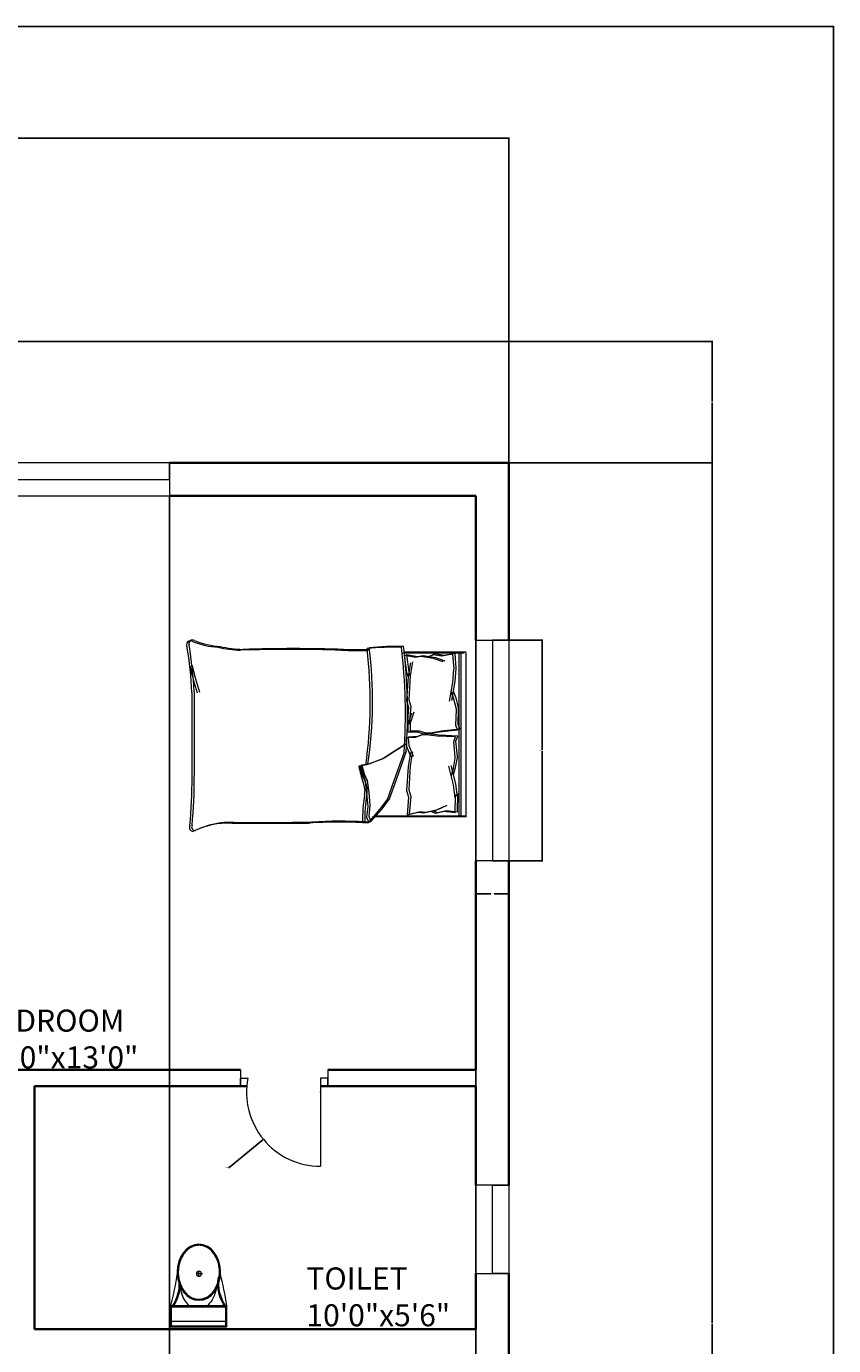
# Model space of a CAD drawing. Units: inches. Extents: x 1902 to 2626, y 1199 to 2408.
# Tile 9 of 9: x 2407 to 2626, y 2049 to 2408. Entities that reach past the tile are written whole.
import ezdxf

# ---------------------------------------------------------------- set-up
doc = ezdxf.new("R2010")
doc.units = ezdxf.units.IN
for name, color, linetype, lineweight in [('A-ANNO-DIMS', 2, 'Continuous', 18), ('A-ANNO-TTLB', 7, 'Continuous', 25), ('A-AREA-IDEN', 7, 'Continuous', 18), ('A-DOOR', 31, 'Continuous', 18), ('A-FLOR-FIXT', 9, 'Continuous', 18), ('A-FURN', 8, 'Continuous', 13), ('A-GLAZ', 181, 'Continuous', 18), ('A-WALL', 7, 'Continuous', 35)]:
    doc.layers.add(name, color=color, linetype=linetype, lineweight=lineweight)
doc.styles.get("Standard").update_dxf_attribs({"font": 'arial.ttf'})
doc.dimstyles.get("Standard").update_dxf_attribs({"dimtxt": 0.18, "dimasz": 0.18, "dimexe": 0.18, "dimexo": 0.0625, "dimgap": 0.09, "dimtad": 0, "dimtih": 1, "dimtoh": 1, "dimdec": 4, "dimzin": 0, "dimdsep": 46, "dimtxsty": 'Standard', "dimcen": 0.09, "dimadec": 0, "dimazin": 0, "dimtfac": 1, "dimtdec": 4, "dimtofl": 0, "dimtmove": 0, "dimatfit": 3, "dimfxl": 1, "dimtolj": 1, "dimtzin": 0, "dimarcsym": 0})

# ---------------------------------------------------------------- blocks, each defined once
blk = doc.blocks.new('A$C31115884')
for p, q in [((283, 498), (223, 498)), ((258, 466), (258, 523)), ((0, 200), (0, 0)), ((520, 200), (0, 200)), ((10, 190), (10, 10)), ((510, 190), (10, 190)), ((510, 10), (510, 190)), ((520, 0), (520, 200)), ((510, 54), (0, 54)), ((10, 10), (510, 10)), ((0, 0), (520, 0))]:
    blk.add_line(p, q)
blk.add_circle((256, 496), 23.6)
for centre, radius, start, end in [((2778, -205), 2807, 165.4549, 171.7133), ((3237, 905), 2807, 188.2867, 194.5451), ((-295, 403), 365, 324.2091, 9.3499), ((-295, 403), 375, 324.2091, 9.3499), ((139, 406), 293, 315.8436, 2.6563), ((806, 403), 375, 179.2036, 215.7909), ((806, 403), 365, 170.6501, 215.7909), ((384, 406), 293, 190.2774, 224.1564)]:
    blk.add_arc(centre, radius, start, end)
blk.add_ellipse((256, 510), major_axis=(0, -261), ratio=0.772727)
blk.add_open_spline([(256, 259), (263, 259), (270, 260), (288, 262), (299, 265), (320, 273), (330, 278), (350, 291), (360, 299), (378, 316), (386, 326), (402, 347), (409, 358), (421, 383), (427, 395), (436, 422), (440, 436), (445, 465), (447, 480), (448, 509), (448, 524), (445, 553), (443, 568), (436, 596), (432, 610), (422, 636), (416, 649), (402, 672), (395, 683), (379, 703), (370, 712), (351, 728), (341, 735), (321, 746), (310, 751), (289, 757), (278, 759), (256, 761), (245, 761), (223, 757), (212, 754), (191, 746), (181, 741), (161, 728), (151, 720), (133, 703), (125, 693), (110, 672), (103, 660), (90, 636), (85, 623), (76, 596), (72, 582), (67, 553), (66, 538), (64, 509), (65, 494), (68, 465), (70, 450), (77, 422), (81, 408), (91, 382), (97, 370), (111, 346), (118, 335), (135, 316), (144, 307), (162, 291), (172, 284), (193, 273), (203, 269), (225, 262), (236, 260), (250, 259), (253, 259), (256, 259)], degree=3, knots=[0, 0, 0, 0, 0.110105, 0.110105, 0.285049, 0.285049, 0.459994, 0.459994, 0.634938, 0.634938, 0.809882, 0.809882, 0.984827, 0.984827, 1.159771, 1.159771, 1.334715, 1.334715, 1.50966, 1.50966, 1.684604, 1.684604, 1.859549, 1.859549, 2.034493, 2.034493, 2.209437, 2.209437, 2.384382, 2.384382, 2.559326, 2.559326, 2.73427, 2.73427, 2.909215, 2.909215, 3.084159, 3.084159, 3.259103, 3.259103, 3.434048, 3.434048, 3.608992, 3.608992, 3.783936, 3.783936, 3.958881, 3.958881, 4.133825, 4.133825, 4.30877, 4.30877, 4.483714, 4.483714, 4.658658, 4.658658, 4.833603, 4.833603, 5.008547, 5.008547, 5.183491, 5.183491, 5.358436, 5.358436, 5.53338, 5.53338, 5.708324, 5.708324, 5.883269, 5.883269, 6.058213, 6.058213, 6.233158, 6.233158, 6.283185, 6.283185, 6.283185, 6.283185])
blk = doc.blocks.new('BED-DOUBLE')
for p, q in [((-0.01, 48.09), (0.59, 48.09)), ((-0.01, 48.09), (-0.01, 3.46)), ((-0.01, 47.87), (24.84, 47.87)), ((-0.01, 47.87), (24.84, 47.87)), ((0.59, 48.09), (25.44, 48.09)), ((0.59, 48.09), (25.44, 48.09)), ((1.43, 3.25), (1.43, 47.87)), ((1.43, 3.25), (1.43, 47.87)), ((2.02, 3.46), (2.02, 48.09)), ((2.02, 3.46), (2.02, 48.09)), ((2.38, 46.8), (2.29, 41.75)), ((2.38, 46.8), (2.29, 41.75)), ((2.38, 46.8), (5.38, 46.44)), ((2.38, 46.8), (5.38, 46.44)), ((2.98, 47.01), (2.89, 41.97)), ((2.98, 47.01), (2.89, 41.96)), ((2.98, 47.01), (5.98, 46.66)), ((2.98, 47.01), (5.98, 46.66)), ((5.38, 46.44), (7.78, 47)), ((5.38, 46.44), (7.78, 47)), ((5.98, 46.66), (8.38, 47.21)), ((5.98, 46.66), (8.38, 47.21)), ((11.04, 46.8), (7.7, 46.05)), ((11.04, 46.8), (7.7, 46.05)), ((7.78, 47), (8.76, 46.52)), ((7.78, 47), (8.76, 46.52)), ((11.64, 47.01), (8.3, 46.26)), ((11.64, 47.01), (8.3, 46.26)), ((8.38, 47.21), (9.35, 46.73)), ((8.38, 47.21), (9.35, 46.73)), ((12.54, 46.62), (11.04, 46.8)), ((12.54, 46.62), (11.04, 46.8)), ((13.14, 46.83), (11.64, 47.01)), ((13.14, 46.83), (11.64, 47.01)), ((15.47, 47.34), (12.54, 46.62)), ((15.47, 47.34), (12.54, 46.62)), ((16.07, 47.56), (13.14, 46.83)), ((16.07, 47.56), (13.14, 46.83)), ((15.09, 42.55), (15.47, 47.34)), ((15.09, 42.55), (15.47, 47.34)), ((15.69, 42.77), (16.07, 47.56)), ((15.69, 42.77), (16.07, 47.56)), ((25.9, 49.37), (22.87, 45.91)), ((25.9, 49.37), (22.87, 45.91)), ((26.5, 49.58), (23.46, 46.12)), ((26.5, 49.58), (23.46, 46.12)), ((27.53, 49.44), (25.9, 49.37, 3.61)), ((27.53, 49.44), (25.9, 49.37, 3.61)), ((26.48, 47.93), (25.9, 49.37)), ((26.48, 47.93), (25.9, 49.37)), ((26.19, 45.04), (26.48, 47.93)), ((26.19, 45.04), (26.48, 47.93)), ((28.13, 49.66), (26.5, 49.58, 3.61)), ((28.13, 49.66), (26.5, 49.58, 3.61)), ((27.08, 48.15), (26.5, 49.58)), ((27.08, 48.15), (26.5, 49.58)), ((26.79, 45.26), (27.08, 48.15)), ((26.79, 45.25), (27.08, 48.15)), ((7.7, 46.05), (5.2, 44.94)), ((7.7, 46.05), (5.2, 44.94)), ((8.3, 46.26), (5.8, 45.16)), ((8.3, 46.26), (5.8, 45.16)), ((20.84, 43.16), (18.97, 37.96)), ((20.84, 43.16), (18.97, 37.96)), ((21.44, 43.38), (19.56, 38.17)), ((21.44, 43.38), (19.56, 38.17)), ((22.87, 45.91), (20.84, 43.16)), ((22.87, 45.91), (20.84, 43.16)), ((23.46, 46.12), (21.44, 43.38)), ((23.46, 46.12), (21.44, 43.38)), ((26.48, 41.43), (26.19, 45.04)), ((26.48, 41.43), (26.19, 45.04)), ((27.08, 41.64), (26.79, 45.26)), ((27.08, 41.64), (26.79, 45.25)), ((2.29, 41.75), (2.37, 42.69)), ((2.29, 41.75), (2.37, 42.69)), ((2.37, 42.69), (2.86, 39.14)), ((2.37, 42.69), (2.86, 39.14)), ((2.89, 41.97), (2.97, 42.9)), ((2.89, 41.96), (2.97, 42.9)), ((2.97, 42.9), (3.46, 39.36)), ((2.97, 42.9), (3.46, 39.35)), ((15.61, 40.72), (15.09, 42.55)), ((15.61, 40.72), (15.09, 42.55)), ((15.21, 34.18), (15.61, 40.72)), ((15.21, 34.18), (15.61, 40.72)), ((16.21, 40.93), (15.69, 42.77)), ((16.21, 40.93), (15.69, 42.77)), ((15.81, 34.39), (16.21, 40.93)), ((15.81, 34.39), (16.21, 40.93)), ((26.91, 38.25), (26.48, 41.43)), ((26.91, 38.24), (26.48, 41.43)), ((27.51, 38.46), (27.08, 41.64)), ((27.51, 38.46), (27.08, 41.64)), ((2.86, 39.14), (4.12, 34.08)), ((2.86, 39.14), (4.12, 34.08)), ((3.42, 36.61), (2.87, 34.68)), ((3.42, 36.61), (2.87, 34.68)), ((3.46, 39.36), (4.72, 34.29)), ((3.46, 39.35), (4.72, 34.29)), ((4.02, 36.82), (3.47, 34.89)), ((4.02, 36.82), (3.47, 34.89)), ((18.97, 37.96), (16.23, 30.17)), ((18.97, 37.96), (16.23, 30.17)), ((19.56, 38.17), (16.82, 30.38)), ((19.56, 38.17), (16.82, 30.38)), ((27.78, 36.37), (26.91, 38.25)), ((27.78, 36.36), (26.91, 38.24)), ((28.38, 36.58), (27.51, 38.46)), ((28.38, 36.58), (27.51, 38.46)), ((28.36, 34.05), (27.78, 36.37)), ((28.36, 34.05), (27.78, 36.36)), ((28.96, 34.26), (28.38, 36.58)), ((28.96, 34.26), (28.38, 36.58)), ((73.99, 14.07), (73.99, 37.05)), ((73.99, 14.07), (73.99, 37.05)), ((74.59, 14.28), (74.59, 37.27)), ((74.59, 14.28), (74.59, 37.27)), ((2.87, 34.68), (2.36, 31.94)), ((2.87, 34.68), (2.36, 31.94)), ((3.47, 34.89), (2.96, 32.16)), ((3.47, 34.89), (2.96, 32.16)), ((14.59, 30.41), (15.21, 34.18)), ((14.59, 30.41), (15.21, 34.18)), ((15.18, 30.62), (15.81, 34.39)), ((15.18, 30.62), (15.81, 34.39)), ((16.82, 28.47), (22.89, 32.38)), ((16.82, 28.47), (22.89, 32.38)), ((22.29, 32.17), (26.48, 33.76)), ((22.29, 32.17), (26.48, 33.76)), ((22.89, 32.38), (27.08, 33.98)), ((22.89, 32.38), (27.08, 33.98)), ((26.48, 33.76), (28.36, 34.05)), ((26.48, 33.76), (28.36, 34.05)), ((27.08, 33.98), (28.96, 34.26)), ((27.08, 33.98), (28.96, 34.26)), ((2.36, 31.94), (2.38, 31.64)), ((2.36, 31.94), (2.38, 31.64)), ((2.38, 31.64), (2.78, 27.51)), ((2.38, 31.64), (2.78, 27.51)), ((2.96, 32.16), (2.98, 31.86)), ((2.96, 32.16), (2.98, 31.86)), ((2.98, 31.86), (3.37, 27.72)), ((2.98, 31.86), (3.37, 27.72)), ((15.63, 28.72), (14.43, 31.58)), ((15.63, 28.72), (14.43, 31.58)), ((16.22, 28.93), (15.02, 31.8)), ((16.22, 28.93), (15.02, 31.8)), ((15.77, 26.43), (15.63, 28.72)), ((15.77, 26.43), (15.63, 28.72)), ((16.37, 26.64), (16.22, 28.93)), ((16.37, 26.64), (16.22, 28.93)), ((16.23, 28.26), (22.29, 32.17)), ((16.23, 28.26), (22.29, 32.17)), ((2.78, 27.51), (2.32, 26.13)), ((2.78, 27.51), (2.32, 26.13)), ((2.32, 26.13), (7.34, 25.9)), ((2.32, 26.13), (7.34, 25.9)), ((3.37, 27.72), (2.92, 26.34)), ((3.37, 27.72), (2.92, 26.34)), ((2.92, 26.34), (7.94, 26.11)), ((2.92, 26.34), (7.94, 26.11)), ((6.74, 24.81), (9.71, 25.35)), ((6.74, 24.81), (9.71, 25.35)), ((7.33, 25.02), (10.3, 25.56)), ((7.33, 25.02), (10.3, 25.56)), ((7.34, 25.9), (10.34, 25.55)), ((7.34, 25.9), (10.34, 25.55)), ((7.94, 26.11), (10.94, 25.76)), ((7.94, 26.11), (10.94, 25.76)), ((9.71, 25.35), (10.92, 25.35)), ((9.71, 25.35), (10.92, 25.35)), ((10.3, 25.56), (11.52, 25.56)), ((10.3, 25.56), (11.52, 25.56)), ((10.34, 25.55), (11.55, 25.62)), ((10.34, 25.55), (11.55, 25.62)), ((10.92, 25.35), (12.68, 24.81)), ((10.92, 25.35), (12.68, 24.81)), ((10.94, 25.76), (12.15, 25.84)), ((10.94, 25.76), (12.15, 25.84)), ((11.52, 25.56), (13.27, 25.02)), ((11.52, 25.56), (13.27, 25.02)), ((11.55, 25.62), (13.27, 26.27)), ((11.55, 25.62), (13.27, 26.27)), ((12.15, 25.84), (13.87, 26.48)), ((12.15, 25.84), (13.87, 26.48)), ((13.27, 26.27), (15.77, 26.43)), ((13.27, 26.27), (15.77, 26.43)), ((13.87, 26.48), (16.37, 26.64)), ((13.87, 26.48), (16.37, 26.64)), ((1.74, 24.27), (6.74, 24.81)), ((1.74, 24.27), (6.74, 24.81)), ((2.28, 22.92), (1.74, 24.27)), ((2.28, 22.92), (1.74, 24.27)), ((2.15, 18.76), (2.28, 22.92)), ((2.15, 18.76), (2.28, 22.92)), ((2.34, 24.48), (7.33, 25.02)), ((2.34, 24.48), (7.33, 25.02)), ((2.88, 23.13), (2.34, 24.48)), ((2.88, 23.13), (2.34, 24.48)), ((2.74, 18.98), (2.88, 23.13)), ((2.74, 18.98), (2.88, 23.13)), ((12.68, 24.81), (15.18, 24.81)), ((12.68, 24.81), (15.18, 24.81)), ((13.27, 25.02), (15.78, 25.02)), ((13.27, 25.02), (15.78, 25.02)), ((15.18, 22.51), (14.16, 19.57)), ((15.18, 22.51), (14.16, 19.57)), ((15.78, 22.72), (14.76, 19.79)), ((15.78, 22.72), (14.76, 19.79)), ((15.09, 18.1), (15.47, 22.9)), ((15.09, 18.1), (15.47, 22.9)), ((15.18, 24.81), (15.18, 22.51)), ((15.18, 24.81), (15.18, 22.51)), ((15.69, 18.32), (16.07, 23.11)), ((15.69, 18.32), (16.07, 23.11)), ((15.78, 25.02), (15.78, 22.72)), ((15.78, 25.02), (15.78, 22.72)), ((2.15, 18.46), (2.15, 18.76)), ((2.15, 18.46), (2.15, 18.76)), ((2.82, 15.76), (2.15, 18.46)), ((2.82, 15.76), (2.15, 18.46)), ((2.74, 18.68), (2.74, 18.98)), ((2.74, 18.68), (2.74, 18.98)), ((3.42, 15.98), (2.74, 18.68)), ((3.42, 15.98), (2.74, 18.68)), ((15.61, 16.27), (15.09, 18.1)), ((15.61, 16.27), (15.09, 18.1)), ((16.21, 16.49), (15.69, 18.32)), ((16.21, 16.49), (15.69, 18.32)), ((3.5, 13.88), (2.82, 15.76)), ((3.5, 13.87), (2.82, 15.76)), ((3.09, 11.31), (4.04, 16.44)), ((3.09, 11.31), (4.04, 16.44)), ((4.09, 14.09), (3.42, 15.98)), ((4.09, 14.09), (3.42, 15.98)), ((3.69, 11.52), (4.63, 16.65)), ((3.69, 11.52), (4.63, 16.65)), ((15.21, 9.73), (15.61, 16.27)), ((15.21, 9.73), (15.61, 16.27)), ((15.81, 9.94), (16.21, 16.49)), ((15.81, 9.94), (16.21, 16.49)), ((2.82, 7.74), (3.09, 11.31)), ((2.82, 7.74), (3.09, 11.31)), ((3.42, 7.95), (3.69, 11.52)), ((3.42, 7.95), (3.69, 11.52)), ((2.8, 7.64), (2.82, 7.74)), ((2.8, 7.64), (2.82, 7.74)), ((3.11, 3.64), (2.8, 7.64)), ((3.11, 3.64), (2.8, 7.64)), ((3.4, 7.86), (3.42, 7.95)), ((3.4, 7.86), (3.42, 7.95)), ((3.71, 3.86), (3.4, 7.86)), ((3.71, 3.86), (3.4, 7.86)), ((14.59, 5.96), (15.21, 9.73)), ((14.59, 5.96), (15.21, 9.73)), ((15.18, 6.18), (15.81, 9.94)), ((15.18, 6.18), (15.81, 9.94)), ((15.21, 9.73), (15.51, 8.67)), ((15.21, 9.73), (15.51, 8.67)), ((15.51, 8.67), (16.19, 3.91)), ((15.51, 8.67), (16.19, 3.91)), ((15.81, 9.94), (16.11, 8.88)), ((15.81, 9.94), (16.11, 8.88)), ((16.11, 8.88), (16.78, 4.12)), ((16.11, 8.88), (16.78, 4.12)), ((3.09, 3.64), (6.06, 4.18)), ((3.09, 3.64), (6.06, 4.18)), ((3.69, 3.85), (6.66, 4.39)), ((3.69, 3.85), (6.66, 4.39)), ((8.36, 4.72), (5.79, 5.67)), ((8.36, 4.72), (5.79, 5.67)), ((6.06, 4.18), (8.49, 3.78)), ((6.06, 4.18), (8.49, 3.78)), ((8.95, 4.93), (6.39, 5.88)), ((8.95, 4.93), (6.39, 5.88)), ((6.66, 4.39), (9.09, 3.99)), ((6.66, 4.39), (9.09, 3.99)), ((11.73, 4.18), (8.36, 4.72)), ((11.73, 4.18), (8.36, 4.72)), ((8.49, 3.78), (9.44, 4.32)), ((8.49, 3.78), (9.44, 4.32)), ((12.33, 4.39), (8.95, 4.93)), ((12.33, 4.39), (8.95, 4.93)), ((9.09, 3.99), (10.03, 4.53)), ((9.09, 3.99), (10.03, 4.53)), ((13.22, 4.45), (11.73, 4.18)), ((13.22, 4.45), (11.73, 4.18)), ((13.81, 4.66), (12.33, 4.39)), ((13.81, 4.66), (12.33, 4.39)), ((16.19, 3.91), (13.22, 4.45)), ((16.19, 3.91), (13.22, 4.45)), ((16.78, 4.12), (13.81, 4.66)), ((16.78, 4.12), (13.81, 4.66)), ((16.91, 3.25), (-0.01, 3.25)), ((16.91, 3.25), (-0.01, 3.25)), ((17.5, 3.46), (0.59, 3.46)), ((17.5, 3.46), (0.59, 3.46))]:
    blk.add_line(p, q)
for centre, radius, start, end in [((64.11, 71.12), 21.54, 267.4714, 296.4681), ((64.11, 71.12), 21.54, 267.4714, 296.4681), ((64.71, 71.33), 21.54, 267.4714, 296.4681), ((64.71, 71.33), 21.54, 267.4714, 296.4681), ((73.64, 50.81), 1.03, 332.6588, 86.02), ((73.64, 50.81), 1.03, 332.6588, 86.02), ((198.21, 38.43), 124.23, 174.4998, 180.6351), ((198.21, 38.43), 124.23, 174.4998, 180.6351), ((74.24, 51.02), 1.03, 332.6588, 86.02), ((74.24, 51.02), 1.03, 332.6588, 86.02), ((198.8, 38.64), 124.23, 174.4998, 180.6351), ((198.8, 38.64), 124.23, 174.4998, 180.6351), ((-6.22, 47.93), 33.79, 349.8763, 2.5657), ((-6.22, 47.93), 33.79, 349.8763, 2.5657), ((33.9, 170.19), 120.92, 266.9791, 273.8365), ((33.9, 170.19), 120.92, 266.9791, 273.8365), ((-5.62, 48.14), 33.79, 349.8763, 2.5657), ((-5.62, 48.14), 33.79, 349.8763, 2.5657), ((34.5, 170.41), 120.92, 266.9791, 273.8365), ((34.5, 170.41), 120.92, 266.9791, 273.8365), ((63.32, -4210.02), 4259.62, 90.00217, 90.28689), ((63.32, -4210.02), 4259.62, 90.00217, 90.28689), ((63.92, -4209.8), 4259.62, 90.00217, 90.28689), ((63.92, -4209.8), 4259.62, 90.00217, 90.28689), ((32.74, 40.85), 5.81, 168.6608, 203.7384), ((32.74, 40.85), 5.81, 168.6608, 203.7384), ((33.33, 41.06), 5.81, 168.6608, 203.7384), ((33.33, 41.06), 5.81, 168.6608, 203.7384), ((1.38, 29.09), 27.69, 10.6617, 19.8806), ((1.38, 29.09), 27.69, 10.6617, 19.8806), ((1.98, 29.31), 27.69, 10.6617, 19.8806), ((1.98, 29.31), 27.69, 10.6617, 19.8806), ((145.95, 16.58), 120.47, 171.7845, 186.9006), ((145.95, 16.58), 120.47, 171.7845, 186.9006), ((146.55, 16.8), 120.47, 171.7845, 186.9006), ((146.55, 16.8), 120.47, 171.7845, 186.9006), ((28.42, 34.21), 0.172, 250.2464, 1.1377), ((28.42, 34.21), 0.172, 250.2464, 1.1377), ((29.01, 34.43), 0.172, 250.2464, 1.1377), ((29.01, 34.43), 0.172, 250.2464, 1.1377), ((169.99, 19.95), 154.04, 176.0865, 186.7821), ((169.99, 19.95), 154.04, 176.0865, 186.7821), ((170.58, 20.16), 154.04, 176.0865, 186.7821), ((170.58, 20.16), 154.04, 176.0865, 186.7821), ((-21.55, -15.86), 99.41, 13.3832, 17.7053), ((-21.55, -15.86), 99.41, 13.3832, 17.7053), ((-22.15, -16.08), 99.41, 13.3832, 17.7053), ((-22.15, -16.08), 99.41, 13.3832, 17.7053), ((187.53, 20.01), 113.69, 182.9958, 189.4091), ((187.53, 20.01), 113.69, 182.9958, 189.4091), ((188.12, 20.22), 113.69, 182.9958, 189.4091), ((188.12, 20.22), 113.69, 182.9958, 189.4091), ((18.76, 79.52), 77.79, 268.7218, 275.604), ((18.76, 79.52), 77.79, 268.7218, 275.604), ((19.36, 79.74), 77.79, 268.7218, 275.604), ((19.36, 79.74), 77.79, 268.7218, 275.604), ((29.1, -156.22), 158.84, 88.4762, 91.0082), ((29.1, -156.22), 158.84, 88.4762, 91.0082), ((29.7, -156), 158.84, 88.4762, 91.0082), ((29.7, -156.01), 158.84, 88.4762, 91.0082), ((47.26, 452.71), 450.36, 268.2277, 271.7185), ((47.26, 452.71), 450.36, 268.2277, 271.7185), ((47.85, 452.92), 450.36, 268.2277, 271.7185), ((47.85, 452.92), 450.36, 268.2277, 271.7185), ((60.24, -25.11), 27.67, 76.0648, 88.9113), ((60.24, -25.11), 27.67, 76.0648, 88.9113), ((60.83, -24.9), 27.67, 76.0648, 88.9113), ((60.83, -24.9), 27.67, 76.0648, 88.9113), ((65.61, -20.22), 22, 67.9751, 86.652), ((65.61, -20.22), 22, 67.9751, 86.652), ((66.21, -20.01), 22, 67.9751, 86.652), ((66.21, -20.01), 22, 67.9751, 86.652), ((74.43, 1.02), 1.02, 236.1736, 23.4781), ((74.43, 1.02), 1.02, 236.1736, 23.4781), ((75.03, 1.23), 1.02, 236.1736, 23.4781), ((75.03, 1.23), 1.02, 236.1736, 23.4781)]:
    blk.add_arc(centre, radius, start, end)
blk = doc.blocks.new('WINDOW-60-A')
for p, q in [((0, 9), (0, 0)), ((60, 9), (0, 9)), ((60, 4.5), (60, 9)), ((60, 9), (60, 0)), ((0, 0), (0, 4.5)), ((0, 4.5), (60, 4.5)), ((0, 0), (60, 0))]:
    blk.add_line(p, q)
blk = doc.blocks.new('WINDOW-60-B')
for p, q in [((0, 60), (9, 60)), ((0, 60), (0, 0)), ((9, 60), (4.5, 60)), ((4.5, 60), (4.5, 0)), ((9, 60), (9, 0)), ((9, 0), (0, 0)), ((4.5, 0), (9, 0))]:
    blk.add_line(p, q)
blk = doc.blocks.new('*D18')
at = {"layer": 'A-ANNO-DIMS', "color": 0, "lineweight": -2, "transparency": 16777216}
for p, q in [((2537.91, 2241.26), (2547.03, 2241.26)), ((2546.85, 2241.08), (2546.85, 2211.44)), ((2546.85, 2181.44), (2546.85, 2211.07)), ((2537.91, 2181.26), (2547.03, 2181.26))]:
    blk.add_line(p, q, dxfattribs=at)
at = {"layer": 'A-ANNO-DIMS', "color": 0, "transparency": 16777216}
for points in [[(2546.82, 2241.08), (2546.88, 2241.08), (2546.85, 2241.26)], [(2546.82, 2181.44), (2546.88, 2181.44), (2546.85, 2181.26)]]:
    blk.add_solid(points, dxfattribs=at)
at = {"layer": 'Defpoints', "color": 0, "transparency": 16777216}
for p in [(2537.85, 2241.26), (2546.85, 2241.26), (2537.85, 2181.26)]:
    blk.add_point(p, dxfattribs=at)
at = {"layer": 'A-ANNO-DIMS', "color": 0, "transparency": 16777216, "insert": (2546.85, 2211.26), "char_height": 0.18, "attachment_point": 5}
blk.add_mtext('\\A1;WIN. B 60 TYP.', dxfattribs=at)
blk = doc.blocks.new('*D19')
at = {"layer": 'A-ANNO-DIMS', "color": 0, "lineweight": -2, "transparency": 16777216}
for p, q in [((2528.85, 2181.19), (2528.85, 2172.08)), ((2537.85, 2181.19), (2537.85, 2172.08)), ((2529.03, 2172.26), (2532.89, 2172.26)), ((2537.67, 2172.26), (2533.81, 2172.26))]:
    blk.add_line(p, q, dxfattribs=at)
at = {"layer": 'A-ANNO-DIMS', "color": 0, "transparency": 16777216}
for points in [[(2529.03, 2172.29), (2529.03, 2172.23), (2528.85, 2172.26)], [(2537.67, 2172.29), (2537.67, 2172.23), (2537.85, 2172.26)]]:
    blk.add_solid(points, dxfattribs=at)
at = {"layer": 'Defpoints', "color": 0, "transparency": 16777216}
for p in [(2528.85, 2181.26), (2537.85, 2181.26), (2537.85, 2172.26)]:
    blk.add_point(p, dxfattribs=at)
at = {"layer": 'A-ANNO-DIMS', "color": 0, "transparency": 16777216, "insert": (2533.35, 2172.26), "char_height": 0.18, "attachment_point": 5}
blk.add_mtext('\\A1;9 TYP.', dxfattribs=at)
blk = doc.blocks.new('*D28')
at = {"layer": 'A-ANNO-DIMS', "color": 0, "lineweight": -2, "transparency": 16777216}
for p, q in [((1999.35, 2289.54), (1999.35, 2377.95)), ((1999.53, 2377.77), (2268.21, 2377.77)), ((2537.67, 2377.77), (2269, 2377.77)), ((2537.85, 2289.54), (2537.85, 2377.95))]:
    blk.add_line(p, q, dxfattribs=at)
at = {"layer": 'A-ANNO-DIMS', "color": 0, "transparency": 16777216}
for points in [[(1999.53, 2377.8), (1999.53, 2377.74), (1999.35, 2377.77)], [(2537.67, 2377.8), (2537.67, 2377.74), (2537.85, 2377.77)]]:
    blk.add_solid(points, dxfattribs=at)
at = {"layer": 'Defpoints', "color": 0, "transparency": 16777216}
for p in [(2537.85, 2377.77), (1999.35, 2289.47), (2537.85, 2289.47)]:
    blk.add_point(p, dxfattribs=at)
at = {"layer": 'A-ANNO-DIMS', "color": 0, "transparency": 16777216, "insert": (2268.6, 2377.77), "char_height": 0.18, "attachment_point": 5}
blk.add_mtext('\\A1;538.5', dxfattribs=at)
blk = doc.blocks.new('*D33')
at = {"layer": 'A-ANNO-DIMS', "color": 0, "lineweight": -2, "transparency": 16777216}
for p, q in [((2537.91, 2289.47), (2593.33, 2289.47)), ((2593.15, 2289.29), (2593.15, 2055.66)), ((2593.15, 1821.65), (2593.15, 2055.29)), ((2528.91, 1821.47), (2593.33, 1821.47))]:
    blk.add_line(p, q, dxfattribs=at)
at = {"layer": 'A-ANNO-DIMS', "color": 0, "transparency": 16777216}
for points in [[(2593.12, 2289.29), (2593.18, 2289.29), (2593.15, 2289.47)], [(2593.12, 1821.65), (2593.18, 1821.65), (2593.15, 1821.47)]]:
    blk.add_solid(points, dxfattribs=at)
at = {"layer": 'Defpoints', "color": 0, "transparency": 16777216}
for p in [(2537.85, 2289.47), (2593.15, 2289.47), (2528.85, 1821.47)]:
    blk.add_point(p, dxfattribs=at)
at = {"layer": 'A-ANNO-DIMS', "color": 0, "transparency": 16777216, "insert": (2593.15, 2055.47), "char_height": 0.18, "attachment_point": 5}
blk.add_mtext('\\A1;468', dxfattribs=at)
blk = doc.blocks.new('*D35')
at = {"layer": 'A-ANNO-DIMS', "color": 0, "lineweight": -2, "transparency": 16777216}
for p, q in [((2341.41, 2322.47), (2593.33, 2322.47)), ((2593.15, 2322.29), (2593.15, 2306.16)), ((2593.15, 2289.65), (2593.15, 2305.79)), ((2537.91, 2289.47), (2593.33, 2289.47))]:
    blk.add_line(p, q, dxfattribs=at)
at = {"layer": 'A-ANNO-DIMS', "color": 0, "transparency": 16777216}
for points in [[(2593.12, 2322.29), (2593.18, 2322.29), (2593.15, 2322.47)], [(2593.12, 2289.65), (2593.18, 2289.65), (2593.15, 2289.47)]]:
    blk.add_solid(points, dxfattribs=at)
at = {"layer": 'Defpoints', "color": 0, "transparency": 16777216}
for p in [(2341.35, 2322.47), (2593.15, 2322.47), (2537.85, 2289.47)]:
    blk.add_point(p, dxfattribs=at)
at = {"layer": 'A-ANNO-DIMS', "color": 0, "transparency": 16777216, "insert": (2593.15, 2305.97), "char_height": 0.18, "attachment_point": 5}
blk.add_mtext('\\A1;33', dxfattribs=at)
blk = doc.blocks.new('*D37')
at = {"layer": 'A-ANNO-DIMS', "color": 0, "lineweight": -2, "transparency": 16777216}
for p, q in [((2445.52, 2280.41), (2445.52, 1198.67)), ((2528.85, 2280.41), (2528.85, 1198.67)), ((2445.7, 1198.85), (2486.79, 1198.85)), ((2528.67, 1198.85), (2487.58, 1198.85))]:
    blk.add_line(p, q, dxfattribs=at)
at = {"layer": 'A-ANNO-DIMS', "color": 0, "transparency": 16777216}
for points in [[(2445.7, 1198.88), (2445.7, 1198.82), (2445.52, 1198.85)], [(2528.67, 1198.88), (2528.67, 1198.82), (2528.85, 1198.85)]]:
    blk.add_solid(points, dxfattribs=at)
at = {"layer": 'Defpoints', "color": 0, "transparency": 16777216}
for p in [(2445.52, 2280.47), (2528.85, 2280.47), (2528.85, 1198.85)]:
    blk.add_point(p, dxfattribs=at)
at = {"layer": 'A-ANNO-DIMS', "color": 0, "transparency": 16777216, "insert": (2487.18, 1198.85), "char_height": 0.18, "attachment_point": 5}
blk.add_mtext('\\A1;83.33', dxfattribs=at)
blk = doc.blocks.new('*D56')
at = {"layer": 'A-ANNO-DIMS', "color": 0, "lineweight": -2, "transparency": 16777216}
for p, q in [((2486.52, 2118.35), (2486.7, 2118.35)), ((2486.61, 2118.26), (2486.61, 2118.44)), ((2461.74, 2097.89), (2470.93, 2105.45)), ((2461.56, 2097.89), (2461.74, 2097.89))]:
    blk.add_line(p, q, dxfattribs=at)
at = {"layer": 'A-ANNO-DIMS', "color": 0, "transparency": 16777216}
blk.add_solid([(2470.91, 2105.47), (2470.95, 2105.42), (2471.07, 2105.56)], dxfattribs=at)
at = {"layer": 'Defpoints', "color": 0, "transparency": 16777216}
for p in [(2486.61, 2118.35), (2471.07, 2105.56)]:
    blk.add_point(p, dxfattribs=at)
at = {"layer": 'A-ANNO-DIMS', "color": 0, "transparency": 16777216, "insert": (2461.01, 2097.89), "char_height": 0.18, "attachment_point": 5}
blk.add_mtext('\\A1;R20.127', dxfattribs=at)

msp = doc.modelspace()

# ---------------------------------------------------------------- linework, layer by layer
at = {"layer": 'A-ANNO-TTLB'}
msp.add_lwpolyline([(1901.6928, 2408.1473), (2626.1646, 2408.1473), (2626.1646, 1206.3103), (1901.6928, 1206.3103)], close=True, dxfattribs=at)
at = {"layer": 'A-DOOR'}
for p, q in [((2464.8563, 2124.4733), (2464.8563, 2119.9733)), ((2488.6076, 2124.4733), (2488.6076, 2119.9733)), ((2464.8563, 2119.9733), (2464.8563, 2122.2233)), ((2464.8563, 2122.2233), (2466.8563, 2122.2233)), ((2488.6076, 2122.2233), (2486.6076, 2122.2233)), ((2486.6076, 2122.2233), (2486.6076, 2098.2233)), ((2488.6076, 2119.9733), (2488.6076, 2122.2233))]:
    msp.add_line(p, q, dxfattribs=at)
msp.add_arc((2486.6076, 2118.3507), 20.1274, 168.906934, 270, dxfattribs=at)
at = {"layer": 'A-GLAZ'}
for p, q in [((2537.8507, 2093.0784), (2528.8507, 2093.0784)), ((2528.8507, 2093.0784), (2528.8507, 2069.0784)), ((2533.3507, 2069.0784), (2533.3507, 2093.0784)), ((2533.3507, 2093.0784), (2537.8507, 2093.0784)), ((2537.8507, 2093.0784), (2537.8507, 2069.0784)), ((2528.8507, 2069.0784), (2537.8507, 2069.0784)), ((2537.8507, 2069.0784), (2533.3507, 2069.0784))]:
    msp.add_line(p, q, dxfattribs=at)
at = {"layer": 'A-WALL'}
for p, q in [((2445.516, 2289.4733), (2537.8507, 2289.4733)), ((2537.8507, 2289.4733), (2537.8507, 2241.2564)), ((2445.516, 2280.4733), (2528.8507, 2280.4733)), ((2528.8507, 2280.4733), (2528.8507, 2241.2564)), ((2528.8507, 2181.2564), (2528.8507, 2124.4733)), ((2537.8507, 2181.2564), (2537.8507, 2119.9733)), ((2336.8507, 2124.4733), (2464.8563, 2124.4733)), ((2488.6076, 2124.4733), (2528.8507, 2124.4733)), ((2537.8507, 2124.4733), (2537.8507, 2093.0784)), ((2408.8507, 2119.9733), (2408.8507, 2053.9733)), ((2408.8507, 2119.9733), (2466.5457, 2119.9733)), ((2486.6076, 2119.9733), (2528.8507, 2119.9733)), ((2528.8507, 2119.9733), (2528.8507, 2093.0784)), ((2528.8507, 2069.0784), (2528.8507, 2053.9733)), ((2537.8507, 2069.0784), (2537.8507, 2028.722)), ((2408.8507, 2053.9733), (2528.8507, 2053.9733))]:
    msp.add_line(p, q, dxfattribs=at)

# ---------------------------------------------------------------- block references
at = {"layer": 'A-FLOR-FIXT', "xscale": -0.0292470664339069, "yscale": 0.0292470664339069, "zscale": 0.0292470664339069}
msp.add_blockref('A$C31115884', (2461.0164, 2054.5045), dxfattribs=at)
at = {"layer": 'A-FURN', "rotation": 180}
msp.add_blockref('BED-DOUBLE', (2526.2281, 2241.3161), dxfattribs=at)
at = {"layer": 'A-GLAZ'}
for name, p in [('WINDOW-60-A', (2385.52, 2280.47)), ('WINDOW-60-B', (2528.85, 2181.26))]:
    msp.add_blockref(name, p, dxfattribs=at)

# ---------------------------------------------------------------- texts
at = {"layer": 'A-AREA-IDEN', "char_height": 6, "attachment_point": 1}
for s, width, insert in [('BEDROOM\\P16\'0"x13\'0"', 174.865201, (2393.4079, 2140.8318)), ('TOILET\\P10\'0"x5\'6"', 104.88024, (2482.7562, 2070.7214))]:
    msp.add_mtext_dynamic_manual_height_columns(s, width=width, gutter_width=12.5, heights=[0], dxfattribs=dict(at, insert=insert))

# ---------------------------------------------------------------- dimensions: what is measured, and where the dimension line sits
at = {"layer": 'A-ANNO-DIMS'}
for base, p1, p2, override, picture, middle in [((2537.8507, 2377.7733), (1999.3507, 2289.4733), (2537.8507, 2289.4733), {"dimdec": 1, "dimlfac": 1, "dimrnd": 0, "dimzin": 0, "dimdsep": 46, "dimlunit": 2}, '*D28', (2268.6007, 2377.7733)), ((2528.8507, 1198.8475), (2445.516, 2280.4733), (2528.8507, 2280.4733), {"dimdec": 2, "dimlfac": 1, "dimrnd": 0, "dimzin": 0, "dimdsep": 46, "dimlunit": 2}, '*D37', (2487.1833, 1198.8475))]:
    dim = msp.add_linear_dim(base=base, p1=p1, p2=p2, dimstyle='Standard', override=override, dxfattribs=at)
    dim.commit()
    dim.dimension.update_dxf_attribs({"geometry": picture, "text_midpoint": middle})
for base, p1, p2, picture, middle in [((2593.1507, 2322.4733), (2537.8507, 2289.4733), (2341.3507, 2322.4733), '*D35', (2593.1507, 2305.9733)), ((2593.1507, 2289.4733), (2528.8507, 1821.4733), (2537.8507, 2289.4733), '*D33', (2593.1507, 2055.4733))]:
    dim = msp.add_linear_dim(base=base, p1=p1, p2=p2, angle=90, dimstyle='Standard', override={"dimdec": 0, "dimlfac": 1, "dimrnd": 0, "dimzin": 0, "dimdsep": 46, "dimlunit": 2}, dxfattribs=at)
    dim.commit()
    dim.dimension.update_dxf_attribs({"geometry": picture, "text_midpoint": middle})
dim = msp.add_linear_dim(base=(2546.8507, 2241.2564), p1=(2537.8507, 2181.2564), p2=(2537.8507, 2241.2564), angle=90, text='WIN. B <> TYP.', dimstyle='Standard', override={"dimdec": 0, "dimlfac": 1, "dimrnd": 0, "dimzin": 0, "dimdsep": 46, "dimlunit": 2}, dxfattribs=at)
dim.commit()
dim.dimension.update_dxf_attribs({"geometry": '*D18', "text_midpoint": (2546.8507, 2211.2564)})
dim = msp.add_linear_dim(base=(2537.8507, 2172.2564), p1=(2528.8507, 2181.2564), p2=(2537.8507, 2181.2564), text='<> TYP.', dimstyle='Standard', override={"dimdec": 0, "dimlfac": 1, "dimrnd": 0, "dimzin": 0, "dimdsep": 46, "dimlunit": 2}, dxfattribs=at)
dim.commit()
dim.dimension.update_dxf_attribs({"geometry": '*D19', "text_midpoint": (2533.3507, 2172.2564)})
dim = msp.add_radius_dim(center=(2486.6076, 2118.3507), mpoint=(2471.0661, 2105.5611), dimstyle='Standard', override={"dimdec": 3, "dimlfac": 1, "dimrnd": 0, "dimzin": 0, "dimdsep": 46, "dimlunit": 2}, dxfattribs=at)
dim.commit()
dim.dimension.update_dxf_attribs({"geometry": '*D56', "text_midpoint": (2461.0115, 2097.8873), "dimtype": 164})

doc.saveas('drawing.dxf')
